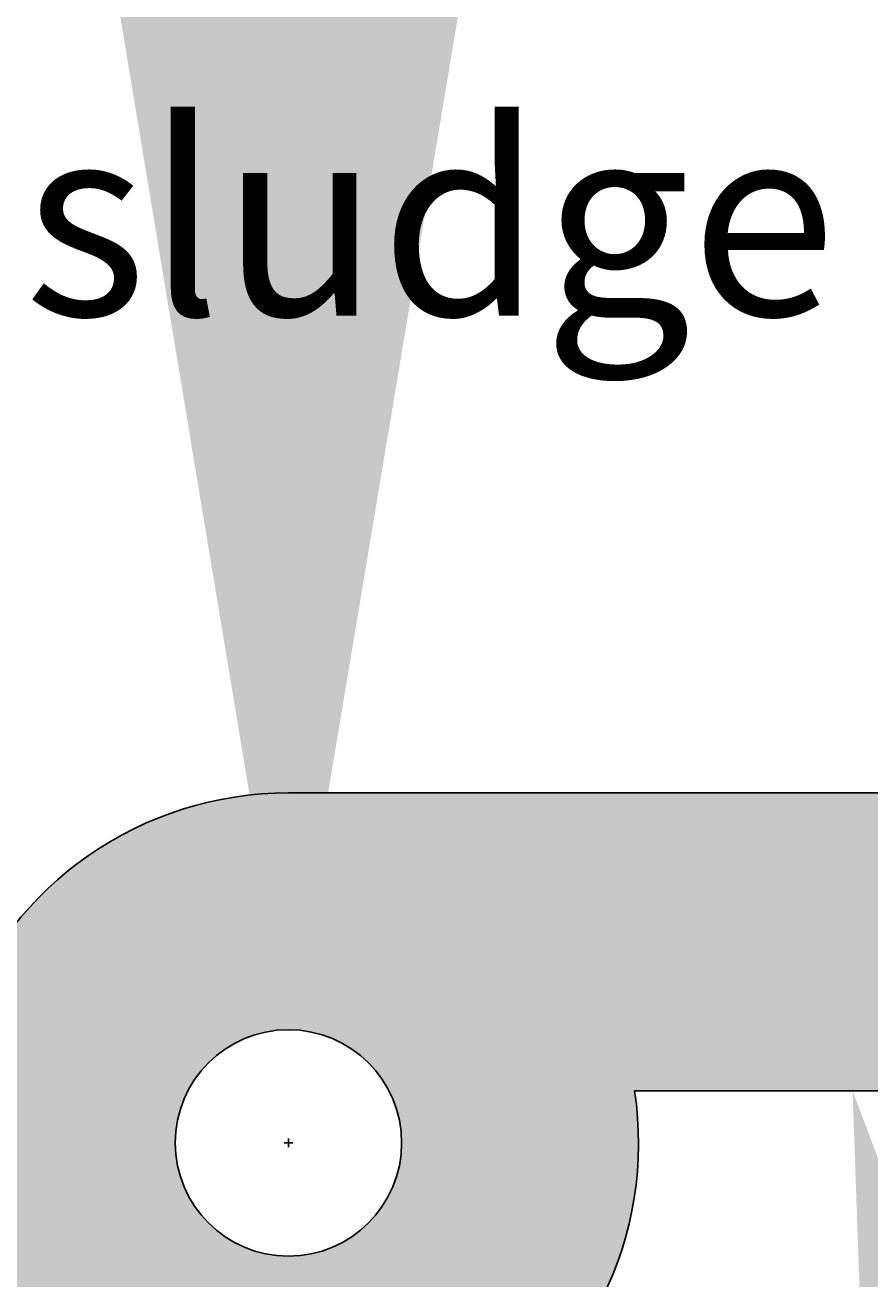
# Model space of a CAD drawing. Units: millimetres. Extents: x -22994 to 29398, y -19990 to 20176.
# Tile 12 of 135: x 41 to 58, y 26 to 52. Entities that reach past the tile are written whole.
import ezdxf
from ezdxf import colors
from ezdxf.entities.mleader import LeaderData, LeaderLine
from ezdxf.math import Vec2, Vec3

# ---------------------------------------------------------------- set-up
doc = ezdxf.new("R2010")
doc.units = ezdxf.units.MM
doc.header["$MEASUREMENT"] = 0
for name, color, linetype, lineweight in [('M-ANNO-TEXT', 7, 'Continuous', 25), ('M-DIMS', 2, 'Continuous', 18), ('M-EQPM', 7, 'Continuous', 25), ('M-EQPM-PATT', 7, 'Continuous', 18)]:
    doc.layers.add(name, color=color, linetype=linetype, lineweight=lineweight)
doc.styles.get("Standard").update_dxf_attribs({"font": 'arial.ttf'})
doc.dimstyles.get("Standard").update_dxf_attribs({"dimtxt": 0.18, "dimasz": 10000, "dimexe": 0.18, "dimexo": 0.0625, "dimgap": 0.09, "dimtad": 0, "dimtih": 1, "dimtoh": 1, "dimdec": 0, "dimzin": 0, "dimdsep": 46, "dimtxsty": 'Standard', "dimcen": 0.09, "dimadec": 0, "dimazin": 0, "dimtfac": 1, "dimtdec": 0, "dimtofl": 0, "dimtmove": 0, "dimatfit": 3, "dimfxl": 1, "dimtolj": 1, "dimtzin": 0, "dimlwd": 30, "dimarcsym": 0})

# ---------------------------------------------------------------- blocks, each defined once
blk = doc.blocks.new('*D2')
at = {"layer": 'Defpoints', "color": 0, "transparency": 16777216}
for p in [(6.677, 10.271), (290.852, 10.271), (290.852, -5.079)]:
    blk.add_point(p, dxfattribs=at)
at = {"layer": 'M-DIMS', "color": 0, "lineweight": -2, "transparency": 16777216}
for p, q in [((6.677, 10.209), (6.677, -5.259)), ((290.852, 10.209), (290.852, -5.259))]:
    blk.add_line(p, q, dxfattribs=at)
at = {"layer": 'M-DIMS', "color": 0, "lineweight": 30, "transparency": 16777216}
for p, q in [((-9993.323, -5.079), (-19993.323, -5.079)), ((10290.852, -5.079), (20290.852, -5.079))]:
    blk.add_line(p, q, dxfattribs=at)
at = {"layer": 'M-DIMS', "color": 0, "transparency": 16777216}
for points in [[(-9993.323, 1661.588), (-9993.323, -1671.745), (6.677, -5.079)], [(10290.852, 1661.588), (10290.852, -1671.745), (290.852, -5.079)]]:
    blk.add_solid(points, dxfattribs=at)
at = {"layer": 'M-DIMS', "color": 0, "transparency": 16777216, "insert": (148.765, -5.079), "char_height": 0.18, "attachment_point": 5}
blk.add_mtext('\\A1;284.2', dxfattribs=at)
blk = doc.blocks.new('*D3')
at = {"layer": 'Defpoints', "color": 0, "transparency": 16777216}
for p in [(110.265, 204.165), (110.265, 176.366), (95.833, 127.967)]:
    blk.add_point(p, dxfattribs=at)
at = {"layer": 'M-DIMS', "color": 0, "lineweight": -2, "transparency": 16777216}
for p, q in [((95.833, 128.03), (95.833, 204.345)), ((110.265, 176.429), (110.265, 204.345))]:
    blk.add_line(p, q, dxfattribs=at)
at = {"layer": 'M-DIMS', "color": 0, "lineweight": 30, "transparency": 16777216}
for p, q in [((-9904.167, 204.165), (-19904.167, 204.165)), ((10110.265, 204.165), (20110.265, 204.165))]:
    blk.add_line(p, q, dxfattribs=at)
at = {"layer": 'M-DIMS', "color": 0, "transparency": 16777216}
for points in [[(-9904.167, 1870.832), (-9904.167, -1462.501), (95.833, 204.165)], [(10110.265, 1870.832), (10110.265, -1462.501), (110.265, 204.165)]]:
    blk.add_solid(points, dxfattribs=at)
at = {"layer": 'M-DIMS', "color": 0, "transparency": 16777216, "insert": (103.049, 204.165), "char_height": 0.18, "attachment_point": 5}
blk.add_mtext('\\A1;14.432', dxfattribs=at)
blk = doc.blocks.new('*D4')
at = {"layer": 'Defpoints', "color": 0, "transparency": 16777216}
for p in [(116.265, 204.165), (110.265, 176.366), (116.265, 176.366)]:
    blk.add_point(p, dxfattribs=at)
at = {"layer": 'M-DIMS', "color": 0, "lineweight": -2, "transparency": 16777216}
for p, q in [((110.265, 176.429), (110.265, 204.345)), ((116.265, 176.429), (116.265, 204.345))]:
    blk.add_line(p, q, dxfattribs=at)
at = {"layer": 'M-DIMS', "color": 0, "lineweight": 30, "transparency": 16777216}
for p, q in [((-9889.735, 204.165), (-19889.735, 204.165)), ((10116.265, 204.165), (20116.265, 204.165))]:
    blk.add_line(p, q, dxfattribs=at)
at = {"layer": 'M-DIMS', "color": 0, "transparency": 16777216}
for points in [[(-9889.735, 1870.832), (-9889.735, -1462.501), (110.265, 204.165)], [(10116.265, 1870.832), (10116.265, -1462.501), (116.265, 204.165)]]:
    blk.add_solid(points, dxfattribs=at)
at = {"layer": 'M-DIMS', "color": 0, "transparency": 16777216, "insert": (113.265, 204.165), "char_height": 0.18, "attachment_point": 5}
blk.add_mtext('\\A1;6', dxfattribs=at)
blk = doc.blocks.new('*D5')
at = {"layer": 'Defpoints', "color": 0, "transparency": 16777216}
for p in [(181.265, 204.165), (116.265, 176.366), (181.265, 176.366)]:
    blk.add_point(p, dxfattribs=at)
at = {"layer": 'M-DIMS', "color": 0, "lineweight": -2, "transparency": 16777216}
for p, q in [((116.265, 176.429), (116.265, 204.345)), ((181.265, 176.429), (181.265, 204.345))]:
    blk.add_line(p, q, dxfattribs=at)
at = {"layer": 'M-DIMS', "color": 0, "lineweight": 30, "transparency": 16777216}
for p, q in [((-9883.735, 204.165), (-19883.735, 204.165)), ((10181.265, 204.165), (20181.265, 204.165))]:
    blk.add_line(p, q, dxfattribs=at)
at = {"layer": 'M-DIMS', "color": 0, "transparency": 16777216}
for points in [[(-9883.735, 1870.832), (-9883.735, -1462.501), (116.265, 204.165)], [(10181.265, 1870.832), (10181.265, -1462.501), (181.265, 204.165)]]:
    blk.add_solid(points, dxfattribs=at)
at = {"layer": 'M-DIMS', "color": 0, "transparency": 16777216, "insert": (148.765, 204.165), "char_height": 0.18, "attachment_point": 5}
blk.add_mtext('\\A1;65', dxfattribs=at)
blk = doc.blocks.new('*D6')
at = {"layer": 'Defpoints', "color": 0, "transparency": 16777216}
for p in [(187.265, 204.165), (181.265, 176.366), (187.265, 176.366)]:
    blk.add_point(p, dxfattribs=at)
at = {"layer": 'M-DIMS', "color": 0, "lineweight": -2, "transparency": 16777216}
for p, q in [((181.265, 176.429), (181.265, 204.345)), ((187.265, 176.429), (187.265, 204.345))]:
    blk.add_line(p, q, dxfattribs=at)
at = {"layer": 'M-DIMS', "color": 0, "lineweight": 30, "transparency": 16777216}
for p, q in [((-9818.735, 204.165), (-19818.735, 204.165)), ((10187.265, 204.165), (20187.265, 204.165))]:
    blk.add_line(p, q, dxfattribs=at)
at = {"layer": 'M-DIMS', "color": 0, "transparency": 16777216}
for points in [[(-9818.735, 1870.832), (-9818.735, -1462.501), (181.265, 204.165)], [(10187.265, 1870.832), (10187.265, -1462.501), (187.265, 204.165)]]:
    blk.add_solid(points, dxfattribs=at)
at = {"layer": 'M-DIMS', "color": 0, "transparency": 16777216, "insert": (184.265, 204.165), "char_height": 0.18, "attachment_point": 5}
blk.add_mtext('\\A1;6', dxfattribs=at)
blk = doc.blocks.new('*D7')
at = {"layer": 'Defpoints', "color": 0, "transparency": 16777216}
for p in [(201.697, 204.165), (187.265, 176.366), (201.697, 127.967)]:
    blk.add_point(p, dxfattribs=at)
at = {"layer": 'M-DIMS', "color": 0, "lineweight": -2, "transparency": 16777216}
for p, q in [((187.265, 176.429), (187.265, 204.345)), ((201.697, 128.03), (201.697, 204.345))]:
    blk.add_line(p, q, dxfattribs=at)
at = {"layer": 'M-DIMS', "color": 0, "lineweight": 30, "transparency": 16777216}
for p, q in [((-9812.735, 204.165), (-19812.735, 204.165)), ((10201.697, 204.165), (20201.697, 204.165))]:
    blk.add_line(p, q, dxfattribs=at)
at = {"layer": 'M-DIMS', "color": 0, "transparency": 16777216}
for points in [[(-9812.735, 1870.832), (-9812.735, -1462.501), (187.265, 204.165)], [(10201.697, 1870.832), (10201.697, -1462.501), (201.697, 204.165)]]:
    blk.add_solid(points, dxfattribs=at)
at = {"layer": 'M-DIMS', "color": 0, "transparency": 16777216, "insert": (194.481, 204.165), "char_height": 0.18, "attachment_point": 5}
blk.add_mtext('\\A1;14.432', dxfattribs=at)
blk = doc.blocks.new('*D8')
at = {"layer": 'Defpoints', "color": 0, "transparency": 16777216}
for p in [(227.648, 204.165), (227.648, 146.73), (201.697, 127.967)]:
    blk.add_point(p, dxfattribs=at)
at = {"layer": 'M-DIMS', "color": 0, "lineweight": -2, "transparency": 16777216}
for p, q in [((201.697, 128.03), (201.697, 204.345)), ((227.648, 146.792), (227.648, 204.345))]:
    blk.add_line(p, q, dxfattribs=at)
at = {"layer": 'M-DIMS', "color": 0, "lineweight": 30, "transparency": 16777216}
for p, q in [((-9798.303, 204.165), (-19798.303, 204.165)), ((10227.648, 204.165), (20227.648, 204.165))]:
    blk.add_line(p, q, dxfattribs=at)
at = {"layer": 'M-DIMS', "color": 0, "transparency": 16777216}
for points in [[(-9798.303, 1870.832), (-9798.303, -1462.501), (201.697, 204.165)], [(10227.648, 1870.832), (10227.648, -1462.501), (227.648, 204.165)]]:
    blk.add_solid(points, dxfattribs=at)
at = {"layer": 'M-DIMS', "color": 0, "transparency": 16777216, "insert": (214.673, 204.165), "char_height": 0.18, "attachment_point": 5}
blk.add_mtext('\\A1;25.95', dxfattribs=at)
blk = doc.blocks.new('*D9')
at = {"layer": 'Defpoints', "color": 0, "transparency": 16777216}
for p in [(187.265, 176.366), (306.202, 176.366), (290.852, 10.271)]:
    blk.add_point(p, dxfattribs=at)
at = {"layer": 'M-DIMS', "color": 0, "lineweight": 30, "transparency": 16777216}
for p, q in [((306.202, 10176.366), (306.202, 20176.366)), ((306.202, -9989.729), (306.202, -19989.729))]:
    blk.add_line(p, q, dxfattribs=at)
at = {"layer": 'M-DIMS', "color": 0, "lineweight": -2, "transparency": 16777216}
for p, q in [((187.327, 176.366), (306.382, 176.366)), ((290.915, 10.271), (306.382, 10.271))]:
    blk.add_line(p, q, dxfattribs=at)
at = {"layer": 'M-DIMS', "color": 0, "transparency": 16777216}
for points in [[(-1360.465, 10176.366), (1972.869, 10176.366), (306.202, 176.366)], [(-1360.465, -9989.729), (1972.869, -9989.729), (306.202, 10.271)]]:
    blk.add_solid(points, dxfattribs=at)
at = {"layer": 'M-DIMS', "color": 0, "transparency": 16777216, "insert": (306.202, 93.319), "char_height": 0.18, "attachment_point": 5}
blk.add_mtext('\\A1;166.1', dxfattribs=at)
blk = doc.blocks.new('*D10')
at = {"layer": 'Defpoints', "color": 0, "transparency": 16777216}
for p in [(125.65, 136.071), (133.346, 136.071), (133.346, -5.079)]:
    blk.add_point(p, dxfattribs=at)
at = {"layer": 'M-DIMS', "color": 0, "lineweight": -2, "transparency": 16777216}
for p, q in [((125.65, 136.009), (125.65, -5.259)), ((133.346, 136.009), (133.346, -5.259))]:
    blk.add_line(p, q, dxfattribs=at)
at = {"layer": 'M-DIMS', "color": 0, "lineweight": 30, "transparency": 16777216}
for p, q in [((-9874.35, -5.079), (-19874.35, -5.079)), ((10133.346, -5.079), (20133.346, -5.079))]:
    blk.add_line(p, q, dxfattribs=at)
at = {"layer": 'M-DIMS', "color": 0, "transparency": 16777216}
for points in [[(-9874.35, 1661.588), (-9874.35, -1671.745), (125.65, -5.079)], [(10133.346, 1661.588), (10133.346, -1671.745), (133.346, -5.079)]]:
    blk.add_solid(points, dxfattribs=at)
at = {"layer": 'M-DIMS', "color": 0, "transparency": 16777216, "insert": (129.498, -5.079), "char_height": 0.18, "attachment_point": 5}
blk.add_mtext('\\A1;7.696', dxfattribs=at)
blk = doc.blocks.new('*D11')
at = {"layer": 'Defpoints', "color": 0, "transparency": 16777216}
for p in [(133.346, 136.071), (135.65, 136.071), (135.65, -5.079)]:
    blk.add_point(p, dxfattribs=at)
at = {"layer": 'M-DIMS', "color": 0, "lineweight": -2, "transparency": 16777216}
for p, q in [((133.346, 136.009), (133.346, -5.259)), ((135.65, 136.009), (135.65, -5.259))]:
    blk.add_line(p, q, dxfattribs=at)
at = {"layer": 'M-DIMS', "color": 0, "lineweight": 30, "transparency": 16777216}
for p, q in [((-9866.654, -5.079), (-19866.654, -5.079)), ((10135.65, -5.079), (20135.65, -5.079))]:
    blk.add_line(p, q, dxfattribs=at)
at = {"layer": 'M-DIMS', "color": 0, "transparency": 16777216}
for points in [[(-9866.654, 1661.588), (-9866.654, -1671.745), (133.346, -5.079)], [(10135.65, 1661.588), (10135.65, -1671.745), (135.65, -5.079)]]:
    blk.add_solid(points, dxfattribs=at)
at = {"layer": 'M-DIMS', "color": 0, "transparency": 16777216, "insert": (134.498, -5.079), "char_height": 0.18, "attachment_point": 5}
blk.add_mtext('\\A1;2.304', dxfattribs=at)
blk = doc.blocks.new('*D12')
at = {"layer": 'Defpoints', "color": 0, "transparency": 16777216}
for p in [(135.65, 136.071), (145.65, 136.071), (145.65, -5.079)]:
    blk.add_point(p, dxfattribs=at)
at = {"layer": 'M-DIMS', "color": 0, "lineweight": -2, "transparency": 16777216}
for p, q in [((135.65, 136.009), (135.65, -5.259)), ((145.65, 136.009), (145.65, -5.259))]:
    blk.add_line(p, q, dxfattribs=at)
at = {"layer": 'M-DIMS', "color": 0, "lineweight": 30, "transparency": 16777216}
for p, q in [((-9864.35, -5.079), (-19864.35, -5.079)), ((10145.65, -5.079), (20145.65, -5.079))]:
    blk.add_line(p, q, dxfattribs=at)
at = {"layer": 'M-DIMS', "color": 0, "transparency": 16777216}
for points in [[(-9864.35, 1661.588), (-9864.35, -1671.745), (135.65, -5.079)], [(10145.65, 1661.588), (10145.65, -1671.745), (145.65, -5.079)]]:
    blk.add_solid(points, dxfattribs=at)
at = {"layer": 'M-DIMS', "color": 0, "transparency": 16777216, "insert": (140.65, -5.079), "char_height": 0.18, "attachment_point": 5}
blk.add_mtext('\\A1;10', dxfattribs=at)
blk = doc.blocks.new('*D13')
at = {"layer": 'Defpoints', "color": 0, "transparency": 16777216}
for p in [(145.65, 136.071), (155.65, 136.071), (155.65, -5.079)]:
    blk.add_point(p, dxfattribs=at)
at = {"layer": 'M-DIMS', "color": 0, "lineweight": -2, "transparency": 16777216}
for p, q in [((145.65, 136.009), (145.65, -5.259)), ((155.65, 136.009), (155.65, -5.259))]:
    blk.add_line(p, q, dxfattribs=at)
at = {"layer": 'M-DIMS', "color": 0, "lineweight": 30, "transparency": 16777216}
for p, q in [((-9854.35, -5.079), (-19854.35, -5.079)), ((10155.65, -5.079), (20155.65, -5.079))]:
    blk.add_line(p, q, dxfattribs=at)
at = {"layer": 'M-DIMS', "color": 0, "transparency": 16777216}
for points in [[(-9854.35, 1661.588), (-9854.35, -1671.745), (145.65, -5.079)], [(10155.65, 1661.588), (10155.65, -1671.745), (155.65, -5.079)]]:
    blk.add_solid(points, dxfattribs=at)
at = {"layer": 'M-DIMS', "color": 0, "transparency": 16777216, "insert": (150.65, -5.079), "char_height": 0.18, "attachment_point": 5}
blk.add_mtext('\\A1;10', dxfattribs=at)
blk = doc.blocks.new('*D14')
at = {"layer": 'Defpoints', "color": 0, "transparency": 16777216}
for p in [(155.65, 136.071), (165.65, 136.071), (165.65, -5.079)]:
    blk.add_point(p, dxfattribs=at)
at = {"layer": 'M-DIMS', "color": 0, "lineweight": -2, "transparency": 16777216}
for p, q in [((155.65, 136.009), (155.65, -5.259)), ((165.65, 136.009), (165.65, -5.259))]:
    blk.add_line(p, q, dxfattribs=at)
at = {"layer": 'M-DIMS', "color": 0, "lineweight": 30, "transparency": 16777216}
for p, q in [((-9844.35, -5.079), (-19844.35, -5.079)), ((10165.65, -5.079), (20165.65, -5.079))]:
    blk.add_line(p, q, dxfattribs=at)
at = {"layer": 'M-DIMS', "color": 0, "transparency": 16777216}
for points in [[(-9844.35, 1661.588), (-9844.35, -1671.745), (155.65, -5.079)], [(10165.65, 1661.588), (10165.65, -1671.745), (165.65, -5.079)]]:
    blk.add_solid(points, dxfattribs=at)
at = {"layer": 'M-DIMS', "color": 0, "transparency": 16777216, "insert": (160.65, -5.079), "char_height": 0.18, "attachment_point": 5}
blk.add_mtext('\\A1;10', dxfattribs=at)
blk = doc.blocks.new('*D15')
at = {"layer": 'Defpoints', "color": 0, "transparency": 16777216}
for p in [(173.346, 154.788), (173.346, 136.071), (306.202, 136.071)]:
    blk.add_point(p, dxfattribs=at)
at = {"layer": 'M-DIMS', "color": 0, "lineweight": 30, "transparency": 16777216}
for p, q in [((306.202, 10154.788), (306.202, 20154.788)), ((306.202, -9863.929), (306.202, -19863.929))]:
    blk.add_line(p, q, dxfattribs=at)
at = {"layer": 'M-DIMS', "color": 0, "lineweight": -2, "transparency": 16777216}
for p, q in [((173.408, 154.788), (306.382, 154.788)), ((173.408, 136.071), (306.382, 136.071))]:
    blk.add_line(p, q, dxfattribs=at)
at = {"layer": 'M-DIMS', "color": 0, "transparency": 16777216}
for points in [[(-1360.465, 10154.788), (1972.869, 10154.788), (306.202, 154.788)], [(-1360.465, -9863.929), (1972.869, -9863.929), (306.202, 136.071)]]:
    blk.add_solid(points, dxfattribs=at)
at = {"layer": 'M-DIMS', "color": 0, "transparency": 16777216, "insert": (306.202, 145.43), "char_height": 0.18, "attachment_point": 5}
blk.add_mtext('\\A1;18.717', dxfattribs=at)
blk = doc.blocks.new('*D16')
at = {"layer": 'Defpoints', "color": 0, "transparency": 16777216}
for p in [(120.17, 204.165), (110.466, 48.035), (120.17, 48.035)]:
    blk.add_point(p, dxfattribs=at)
at = {"layer": 'M-DIMS', "color": 0, "lineweight": -2, "transparency": 16777216}
for p, q in [((110.466, 48.097), (110.466, 204.345)), ((120.17, 48.097), (120.17, 204.345))]:
    blk.add_line(p, q, dxfattribs=at)
at = {"layer": 'M-DIMS', "color": 0, "lineweight": 30, "transparency": 16777216}
for p, q in [((-9889.534, 204.165), (-19889.534, 204.165)), ((10120.17, 204.165), (20120.17, 204.165))]:
    blk.add_line(p, q, dxfattribs=at)
at = {"layer": 'M-DIMS', "color": 0, "transparency": 16777216}
for points in [[(-9889.534, 1870.832), (-9889.534, -1462.501), (110.466, 204.165)], [(10120.17, 1870.832), (10120.17, -1462.501), (120.17, 204.165)]]:
    blk.add_solid(points, dxfattribs=at)
at = {"layer": 'M-DIMS', "color": 0, "transparency": 16777216, "insert": (115.318, 204.165), "char_height": 0.18, "attachment_point": 5}
blk.add_mtext('\\A1;9.704', dxfattribs=at)
blk = doc.blocks.new('*D17')
at = {"layer": 'Defpoints', "color": 0, "transparency": 16777216}
for p in [(126.17, 204.165), (120.17, 48.035), (126.17, 48.035)]:
    blk.add_point(p, dxfattribs=at)
at = {"layer": 'M-DIMS', "color": 0, "lineweight": -2, "transparency": 16777216}
for p, q in [((120.17, 48.097), (120.17, 204.345)), ((126.17, 48.097), (126.17, 204.345))]:
    blk.add_line(p, q, dxfattribs=at)
at = {"layer": 'M-DIMS', "color": 0, "lineweight": 30, "transparency": 16777216}
for p, q in [((-9879.83, 204.165), (-19879.83, 204.165)), ((10126.17, 204.165), (20126.17, 204.165))]:
    blk.add_line(p, q, dxfattribs=at)
at = {"layer": 'M-DIMS', "color": 0, "transparency": 16777216}
for points in [[(-9879.83, 1870.832), (-9879.83, -1462.501), (120.17, 204.165)], [(10126.17, 1870.832), (10126.17, -1462.501), (126.17, 204.165)]]:
    blk.add_solid(points, dxfattribs=at)
at = {"layer": 'M-DIMS', "color": 0, "transparency": 16777216, "insert": (123.17, 204.165), "char_height": 0.18, "attachment_point": 5}
blk.add_mtext('\\A1;6', dxfattribs=at)
blk = doc.blocks.new('*D18')
at = {"layer": 'Defpoints', "color": 0, "transparency": 16777216}
for p in [(132.17, 204.165), (126.17, 48.035), (132.17, 48.035)]:
    blk.add_point(p, dxfattribs=at)
at = {"layer": 'M-DIMS', "color": 0, "lineweight": -2, "transparency": 16777216}
for p, q in [((126.17, 48.097), (126.17, 204.345)), ((132.17, 48.097), (132.17, 204.345))]:
    blk.add_line(p, q, dxfattribs=at)
at = {"layer": 'M-DIMS', "color": 0, "lineweight": 30, "transparency": 16777216}
for p, q in [((-9873.83, 204.165), (-19873.83, 204.165)), ((10132.17, 204.165), (20132.17, 204.165))]:
    blk.add_line(p, q, dxfattribs=at)
at = {"layer": 'M-DIMS', "color": 0, "transparency": 16777216}
for points in [[(-9873.83, 1870.832), (-9873.83, -1462.501), (126.17, 204.165)], [(10132.17, 1870.832), (10132.17, -1462.501), (132.17, 204.165)]]:
    blk.add_solid(points, dxfattribs=at)
at = {"layer": 'M-DIMS', "color": 0, "transparency": 16777216, "insert": (129.17, 204.165), "char_height": 0.18, "attachment_point": 5}
blk.add_mtext('\\A1;6', dxfattribs=at)
blk = doc.blocks.new('*D19')
at = {"layer": 'Defpoints', "color": 0, "transparency": 16777216}
for p in [(138.17, 204.165), (132.17, 48.035), (138.17, 48.035)]:
    blk.add_point(p, dxfattribs=at)
at = {"layer": 'M-DIMS', "color": 0, "lineweight": -2, "transparency": 16777216}
for p, q in [((132.17, 48.097), (132.17, 204.345)), ((138.17, 48.097), (138.17, 204.345))]:
    blk.add_line(p, q, dxfattribs=at)
at = {"layer": 'M-DIMS', "color": 0, "lineweight": 30, "transparency": 16777216}
for p, q in [((-9867.83, 204.165), (-19867.83, 204.165)), ((10138.17, 204.165), (20138.17, 204.165))]:
    blk.add_line(p, q, dxfattribs=at)
at = {"layer": 'M-DIMS', "color": 0, "transparency": 16777216}
for points in [[(-9867.83, 1870.832), (-9867.83, -1462.501), (132.17, 204.165)], [(10138.17, 1870.832), (10138.17, -1462.501), (138.17, 204.165)]]:
    blk.add_solid(points, dxfattribs=at)
at = {"layer": 'M-DIMS', "color": 0, "transparency": 16777216, "insert": (135.17, 204.165), "char_height": 0.18, "attachment_point": 5}
blk.add_mtext('\\A1;6', dxfattribs=at)
blk = doc.blocks.new('*D20')
at = {"layer": 'Defpoints', "color": 0, "transparency": 16777216}
for p in [(144.17, 204.165), (138.17, 48.035), (144.17, 48.035)]:
    blk.add_point(p, dxfattribs=at)
at = {"layer": 'M-DIMS', "color": 0, "lineweight": -2, "transparency": 16777216}
for p, q in [((138.17, 48.097), (138.17, 204.345)), ((144.17, 48.097), (144.17, 204.345))]:
    blk.add_line(p, q, dxfattribs=at)
at = {"layer": 'M-DIMS', "color": 0, "lineweight": 30, "transparency": 16777216}
for p, q in [((-9861.83, 204.165), (-19861.83, 204.165)), ((10144.17, 204.165), (20144.17, 204.165))]:
    blk.add_line(p, q, dxfattribs=at)
at = {"layer": 'M-DIMS', "color": 0, "transparency": 16777216}
for points in [[(-9861.83, 1870.832), (-9861.83, -1462.501), (138.17, 204.165)], [(10144.17, 1870.832), (10144.17, -1462.501), (144.17, 204.165)]]:
    blk.add_solid(points, dxfattribs=at)
at = {"layer": 'M-DIMS', "color": 0, "transparency": 16777216, "insert": (141.17, 204.165), "char_height": 0.18, "attachment_point": 5}
blk.add_mtext('\\A1;6', dxfattribs=at)
blk = doc.blocks.new('*D21')
at = {"layer": 'Defpoints', "color": 0, "transparency": 16777216}
for p in [(149.116, 204.165), (144.17, 48.035), (149.116, 48.035)]:
    blk.add_point(p, dxfattribs=at)
at = {"layer": 'M-DIMS', "color": 0, "lineweight": -2, "transparency": 16777216}
for p, q in [((144.17, 48.097), (144.17, 204.345)), ((149.116, 48.097), (149.116, 204.345))]:
    blk.add_line(p, q, dxfattribs=at)
at = {"layer": 'M-DIMS', "color": 0, "lineweight": 30, "transparency": 16777216}
for p, q in [((-9855.83, 204.165), (-19855.83, 204.165)), ((10149.116, 204.165), (20149.116, 204.165))]:
    blk.add_line(p, q, dxfattribs=at)
at = {"layer": 'M-DIMS', "color": 0, "transparency": 16777216}
for points in [[(-9855.83, 1870.832), (-9855.83, -1462.501), (144.17, 204.165)], [(10149.116, 1870.832), (10149.116, -1462.501), (149.116, 204.165)]]:
    blk.add_solid(points, dxfattribs=at)
at = {"layer": 'M-DIMS', "color": 0, "transparency": 16777216, "insert": (146.643, 204.165), "char_height": 0.18, "attachment_point": 5}
blk.add_mtext('\\A1;4.945', dxfattribs=at)
blk = doc.blocks.new('*D22')
at = {"layer": 'Defpoints', "color": 0, "transparency": 16777216}
for p in [(149.116, 30.99), (155.116, 30.99), (155.116, -5.079)]:
    blk.add_point(p, dxfattribs=at)
at = {"layer": 'M-DIMS', "color": 0, "lineweight": -2, "transparency": 16777216}
for p, q in [((149.116, 30.927), (149.116, -5.259)), ((155.116, 30.927), (155.116, -5.259))]:
    blk.add_line(p, q, dxfattribs=at)
at = {"layer": 'M-DIMS', "color": 0, "lineweight": 30, "transparency": 16777216}
for p, q in [((-9850.884, -5.079), (-19850.884, -5.079)), ((10155.116, -5.079), (20155.116, -5.079))]:
    blk.add_line(p, q, dxfattribs=at)
at = {"layer": 'M-DIMS', "color": 0, "transparency": 16777216}
for points in [[(-9850.884, 1661.588), (-9850.884, -1671.745), (149.116, -5.079)], [(10155.116, 1661.588), (10155.116, -1671.745), (155.116, -5.079)]]:
    blk.add_solid(points, dxfattribs=at)
at = {"layer": 'M-DIMS', "color": 0, "transparency": 16777216, "insert": (152.116, -5.079), "char_height": 0.18, "attachment_point": 5}
blk.add_mtext('\\A1;6', dxfattribs=at)
blk = doc.blocks.new('*D23')
at = {"layer": 'Defpoints', "color": 0, "transparency": 16777216}
for p in [(155.116, 30.99), (161.116, 30.99), (161.116, -5.079)]:
    blk.add_point(p, dxfattribs=at)
at = {"layer": 'M-DIMS', "color": 0, "lineweight": -2, "transparency": 16777216}
for p, q in [((155.116, 30.927), (155.116, -5.259)), ((161.116, 30.927), (161.116, -5.259))]:
    blk.add_line(p, q, dxfattribs=at)
at = {"layer": 'M-DIMS', "color": 0, "lineweight": 30, "transparency": 16777216}
for p, q in [((-9844.884, -5.079), (-19844.884, -5.079)), ((10161.116, -5.079), (20161.116, -5.079))]:
    blk.add_line(p, q, dxfattribs=at)
at = {"layer": 'M-DIMS', "color": 0, "transparency": 16777216}
for points in [[(-9844.884, 1661.588), (-9844.884, -1671.745), (155.116, -5.079)], [(10161.116, 1661.588), (10161.116, -1671.745), (161.116, -5.079)]]:
    blk.add_solid(points, dxfattribs=at)
at = {"layer": 'M-DIMS', "color": 0, "transparency": 16777216, "insert": (158.116, -5.079), "char_height": 0.18, "attachment_point": 5}
blk.add_mtext('\\A1;6', dxfattribs=at)
blk = doc.blocks.new('*D24')
at = {"layer": 'Defpoints', "color": 0, "transparency": 16777216}
for p in [(161.116, 30.99), (166.439, 30.99), (166.439, -5.079)]:
    blk.add_point(p, dxfattribs=at)
at = {"layer": 'M-DIMS', "color": 0, "lineweight": -2, "transparency": 16777216}
for p, q in [((161.116, 30.927), (161.116, -5.259)), ((166.439, 30.927), (166.439, -5.259))]:
    blk.add_line(p, q, dxfattribs=at)
at = {"layer": 'M-DIMS', "color": 0, "lineweight": 30, "transparency": 16777216}
for p, q in [((-9838.884, -5.079), (-19838.884, -5.079)), ((10166.439, -5.079), (20166.439, -5.079))]:
    blk.add_line(p, q, dxfattribs=at)
at = {"layer": 'M-DIMS', "color": 0, "transparency": 16777216}
for points in [[(-9838.884, 1661.588), (-9838.884, -1671.745), (161.116, -5.079)], [(10166.439, 1661.588), (10166.439, -1671.745), (166.439, -5.079)]]:
    blk.add_solid(points, dxfattribs=at)
at = {"layer": 'M-DIMS', "color": 0, "transparency": 16777216, "insert": (163.777, -5.079), "char_height": 0.18, "attachment_point": 5}
blk.add_mtext('\\A1;5.323', dxfattribs=at)
blk = doc.blocks.new('*D25')
at = {"layer": 'Defpoints', "color": 0, "transparency": 16777216}
for p in [(166.439, 30.99), (172.439, 30.99), (172.439, -5.079)]:
    blk.add_point(p, dxfattribs=at)
at = {"layer": 'M-DIMS', "color": 0, "lineweight": -2, "transparency": 16777216}
for p, q in [((166.439, 30.927), (166.439, -5.259)), ((172.439, 30.927), (172.439, -5.259))]:
    blk.add_line(p, q, dxfattribs=at)
at = {"layer": 'M-DIMS', "color": 0, "lineweight": 30, "transparency": 16777216}
for p, q in [((-9833.561, -5.079), (-19833.561, -5.079)), ((10172.439, -5.079), (20172.439, -5.079))]:
    blk.add_line(p, q, dxfattribs=at)
at = {"layer": 'M-DIMS', "color": 0, "transparency": 16777216}
for points in [[(-9833.561, 1661.588), (-9833.561, -1671.745), (166.439, -5.079)], [(10172.439, 1661.588), (10172.439, -1671.745), (172.439, -5.079)]]:
    blk.add_solid(points, dxfattribs=at)
at = {"layer": 'M-DIMS', "color": 0, "transparency": 16777216, "insert": (169.439, -5.079), "char_height": 0.18, "attachment_point": 5}
blk.add_mtext('\\A1;6', dxfattribs=at)
blk = doc.blocks.new('*D26')
at = {"layer": 'Defpoints', "color": 0, "transparency": 16777216}
for p in [(172.439, 30.99), (178.439, 30.99), (178.439, -5.079)]:
    blk.add_point(p, dxfattribs=at)
at = {"layer": 'M-DIMS', "color": 0, "lineweight": -2, "transparency": 16777216}
for p, q in [((172.439, 30.927), (172.439, -5.259)), ((178.439, 30.927), (178.439, -5.259))]:
    blk.add_line(p, q, dxfattribs=at)
at = {"layer": 'M-DIMS', "color": 0, "lineweight": 30, "transparency": 16777216}
for p, q in [((-9827.561, -5.079), (-19827.561, -5.079)), ((10178.439, -5.079), (20178.439, -5.079))]:
    blk.add_line(p, q, dxfattribs=at)
at = {"layer": 'M-DIMS', "color": 0, "transparency": 16777216}
for points in [[(-9827.561, 1661.588), (-9827.561, -1671.745), (172.439, -5.079)], [(10178.439, 1661.588), (10178.439, -1671.745), (178.439, -5.079)]]:
    blk.add_solid(points, dxfattribs=at)
at = {"layer": 'M-DIMS', "color": 0, "transparency": 16777216, "insert": (175.439, -5.079), "char_height": 0.18, "attachment_point": 5}
blk.add_mtext('\\A1;6', dxfattribs=at)
blk = doc.blocks.new('*D27')
at = {"layer": 'Defpoints', "color": 0, "transparency": 16777216}
for p in [(178.439, 30.99), (188.117, 30.99), (188.117, -5.079)]:
    blk.add_point(p, dxfattribs=at)
at = {"layer": 'M-DIMS', "color": 0, "lineweight": -2, "transparency": 16777216}
for p, q in [((178.439, 30.927), (178.439, -5.259)), ((188.117, 30.927), (188.117, -5.259))]:
    blk.add_line(p, q, dxfattribs=at)
at = {"layer": 'M-DIMS', "color": 0, "lineweight": 30, "transparency": 16777216}
for p, q in [((-9821.561, -5.079), (-19821.561, -5.079)), ((10188.117, -5.079), (20188.117, -5.079))]:
    blk.add_line(p, q, dxfattribs=at)
at = {"layer": 'M-DIMS', "color": 0, "transparency": 16777216}
for points in [[(-9821.561, 1661.588), (-9821.561, -1671.745), (178.439, -5.079)], [(10188.117, 1661.588), (10188.117, -1671.745), (188.117, -5.079)]]:
    blk.add_solid(points, dxfattribs=at)
at = {"layer": 'M-DIMS', "color": 0, "transparency": 16777216, "insert": (183.278, -5.079), "char_height": 0.18, "attachment_point": 5}
blk.add_mtext('\\A1;9.679', dxfattribs=at)
blk = doc.blocks.new('*D28')
at = {"layer": 'Defpoints', "color": 0, "transparency": 16777216}
for p in [(188.117, 48.035), (306.202, 48.035), (188.117, 30.99)]:
    blk.add_point(p, dxfattribs=at)
at = {"layer": 'M-DIMS', "color": 0, "lineweight": 30, "transparency": 16777216}
for p, q in [((306.202, 10048.035), (306.202, 20048.035)), ((306.202, -9969.01), (306.202, -19969.01))]:
    blk.add_line(p, q, dxfattribs=at)
at = {"layer": 'M-DIMS', "color": 0, "lineweight": -2, "transparency": 16777216}
for p, q in [((188.18, 48.035), (306.382, 48.035)), ((188.18, 30.99), (306.382, 30.99))]:
    blk.add_line(p, q, dxfattribs=at)
at = {"layer": 'M-DIMS', "color": 0, "transparency": 16777216}
for points in [[(-1360.465, 10048.035), (1972.869, 10048.035), (306.202, 48.035)], [(-1360.465, -9969.01), (1972.869, -9969.01), (306.202, 30.99)]]:
    blk.add_solid(points, dxfattribs=at)
at = {"layer": 'M-DIMS', "color": 0, "transparency": 16777216, "insert": (306.202, 39.512), "char_height": 0.18, "attachment_point": 5}
blk.add_mtext('\\A1;17.045', dxfattribs=at)
blk = doc.blocks.new('*D29')
at = {"layer": 'Defpoints', "color": 0, "transparency": 16777216}
for p in [(36.801, 80.045), (64.03, 80.045)]:
    blk.add_point(p, dxfattribs=at)
at = {"layer": 'M-DIMS', "color": 0, "lineweight": -2, "transparency": 16777216}
for p, q in [((50.415, 79.955), (50.415, 80.135)), ((50.325, 80.045), (50.505, 80.045))]:
    blk.add_line(p, q, dxfattribs=at)
at = {"layer": 'M-DIMS', "color": 0, "lineweight": 30, "transparency": 16777216}
blk.add_line((20064.03, 80.03), (10064.03, 80.038), dxfattribs=at)
at = {"layer": 'M-DIMS', "color": 0, "transparency": 16777216}
blk.add_solid([(10064.031, 1746.704), (10064.028, -1586.629), (64.03, 80.045)], dxfattribs=at)
at = {"layer": 'M-DIMS', "color": 0, "transparency": 16777216, "insert": (20064.521, 80.03), "char_height": 0.18, "attachment_point": 5}
blk.add_mtext('\\A1;∅27.23', dxfattribs=at)
blk = doc.blocks.new('*D32')
at = {"layer": 'Defpoints', "color": 0, "transparency": 16777216}
for p in [(57.164, 118.614), (52.413, 113.093)]:
    blk.add_point(p, dxfattribs=at)
at = {"layer": 'M-DIMS', "color": 0, "lineweight": -2, "transparency": 16777216}
for p, q in [((57.074, 118.614), (57.254, 118.614)), ((57.164, 118.524), (57.164, 118.704))]:
    blk.add_line(p, q, dxfattribs=at)
at = {"layer": 'M-DIMS', "color": 0, "lineweight": 30, "transparency": 16777216}
for p, q in [((-12992.534, -15047.031), (-6470.06, -7466.969)), ((-22992.534, -15047.031), (-12992.534, -15047.031))]:
    blk.add_line(p, q, dxfattribs=at)
at = {"layer": 'M-DIMS', "color": 0, "transparency": 16777216}
blk.add_solid([(-7733.404, -6379.89), (-5206.717, -8554.048), (52.413, 113.093)], dxfattribs=at)
at = {"layer": 'M-DIMS', "color": 0, "transparency": 16777216, "insert": (-22993.208, -15047.031), "char_height": 0.18, "attachment_point": 5}
blk.add_mtext('\\A1;2X R7.284', dxfattribs=at)
blk = doc.blocks.new('*D36')
at = {"layer": 'Defpoints', "color": 0, "transparency": 16777216}
for p in [(46.39, 31.303), (46.387, 26.593)]:
    blk.add_point(p, dxfattribs=at)
at = {"layer": 'M-DIMS', "color": 0, "lineweight": 30, "transparency": 16777216}
for p, q in [((57.15, 20031.301), (51.77, 10031.302)), ((10057.15, 20031.301), (57.15, 20031.301))]:
    blk.add_line(p, q, dxfattribs=at)
at = {"layer": 'M-DIMS', "color": 0, "lineweight": -2, "transparency": 16777216}
for p, q in [((46.389, 28.858), (46.389, 29.038)), ((46.299, 28.948), (46.479, 28.948))]:
    blk.add_line(p, q, dxfattribs=at)
at = {"layer": 'M-DIMS', "color": 0, "transparency": 16777216}
blk.add_solid([(-1614.896, 10032.199), (1718.436, 10030.405), (46.39, 31.303)], dxfattribs=at)
at = {"layer": 'M-DIMS', "color": 0, "transparency": 16777216, "insert": (10057.554, 20031.301), "char_height": 0.18, "attachment_point": 5}
blk.add_mtext('\\A1;∅4.71', dxfattribs=at)
blk = doc.blocks.new('*D37')
at = {"layer": 'Defpoints', "color": 0, "transparency": 16777216}
for p in [(54.834, 118.615), (59.494, 118.614)]:
    blk.add_point(p, dxfattribs=at)
at = {"layer": 'M-DIMS', "color": 0, "lineweight": -2, "transparency": 16777216}
for p, q in [((57.074, 118.614), (57.254, 118.614)), ((57.164, 118.524), (57.164, 118.704))]:
    blk.add_line(p, q, dxfattribs=at)
at = {"layer": 'M-DIMS', "color": 0, "lineweight": 30, "transparency": 16777216}
blk.add_line((20059.493, 116.253), (10059.494, 117.434), dxfattribs=at)
at = {"layer": 'M-DIMS', "color": 0, "transparency": 16777216}
blk.add_solid([(10059.69, 1784.1), (10059.297, -1549.233), (59.494, 118.614)], dxfattribs=at)
at = {"layer": 'M-DIMS', "color": 0, "transparency": 16777216, "insert": (20059.985, 116.253), "char_height": 0.18, "attachment_point": 5}
blk.add_mtext('\\A1;∅4.659', dxfattribs=at)

msp = doc.modelspace()

# ---------------------------------------------------------------- hatches: boundary and pattern name
at = {"layer": 'M-EQPM-PATT'}
h = msp.add_hatch(color=256, dxfattribs=at)
h.set_gradient(color1=(242, 103, 34), color2=(242, 103, 34), tint=1, name='CYLINDER')
h.paths.add_polyline_path([(53.5912, 30.0354), (64.8905, 30.0354), (64.8905, 36.2325), (46.3887, 36.2325, 2.6954641)])
h.paths.add_polyline_path([(44.0337, 28.9485, -1), (48.7438, 28.9485, -1)], flags=16)
h.paths.add_polyline_path([(75.6657, 119.7012), (75.6657, 125.8983), (57.1639, 125.8983, 2.6954641), (64.3664, 119.7012)])
h.paths.add_polyline_path([(59.4936, 118.6143, -1), (54.8343, 118.6143, -1)], flags=16)

# ---------------------------------------------------------------- linework, layer by layer
at = {"layer": 'M-EQPM'}
for p, q in [((46.3887, 36.2325), (64.8905, 36.2325)), ((64.8905, 30.0354), (53.5912, 30.0354))]:
    msp.add_line(p, q, dxfattribs=at)
msp.add_circle((46.3887, 28.9485), 2.355, dxfattribs=at)
msp.add_arc((46.3887, 28.9485), 7.284, 90, 8.58187, dxfattribs=at)

# ---------------------------------------------------------------- texts
at = {"layer": 'M-ANNO-TEXT', "insert": (40.8825, 50.1638), "char_height": 4, "attachment_point": 1}
msp.add_mtext_dynamic_manual_height_columns('sludge', width=25.210711, gutter_width=1, heights=[0], dxfattribs=at)

# ---------------------------------------------------------------- dimensions: what is measured, and where the dimension line sits
at = {"layer": 'M-DIMS'}
for base, p1, p2, override, picture, middle in [((306.202, 176.3662), (290.852, 10.2713), (187.2647, 176.3662), {"dimdec": 1, "dimlfac": 1, "dimrnd": 0, "dimzin": 0, "dimdsep": 46, "dimlunit": 2}, '*D9', (306.202, 93.3187)), ((306.202, 136.0713), (173.3459, 154.788), (173.3459, 136.0713), {"dimdec": 3, "dimlfac": 1, "dimrnd": 0, "dimzin": 0, "dimdsep": 46, "dimlunit": 2}, '*D15', (306.202, 145.4297)), ((306.202, 48.0349), (188.1175, 30.9895), (188.1175, 48.0349), {"dimdec": 3, "dimlfac": 1, "dimrnd": 0, "dimzin": 0, "dimdsep": 46, "dimlunit": 2}, '*D28', (306.202, 39.5122))]:
    dim = msp.add_linear_dim(base=base, p1=p1, p2=p2, angle=90, dimstyle='Standard', override=override, dxfattribs=at)
    dim.commit()
    dim.dimension.update_dxf_attribs({"geometry": picture, "text_midpoint": middle})
dim = msp.add_diameter_dim_2p(p1=(46.3875, 26.5934), p2=(46.39, 31.3035), dimstyle='Standard', override={"dimdec": 2, "dimlfac": 1, "dimrnd": 0, "dimzin": 0, "dimdsep": 46, "dimlunit": 2}, dxfattribs=at)
dim.commit()
dim.dimension.update_dxf_attribs({"geometry": '*D36', "text_midpoint": (10057.5542, 20031.3006), "dimtype": 163})
for base, p1, p2, override, picture, middle in [((110.2647, 204.1654), (95.8327, 127.967), (110.2647, 176.3662), {"dimdec": 3, "dimlfac": 1, "dimrnd": 0, "dimzin": 0, "dimdsep": 46, "dimlunit": 2}, '*D3', (103.0487, 204.1654)), ((116.2647, 204.1654), (110.2647, 176.3662), (116.2647, 176.3662), {"dimdec": 0, "dimlfac": 1, "dimrnd": 0, "dimzin": 0, "dimdsep": 46, "dimlunit": 2}, '*D4', (113.2647, 204.1654)), ((120.1702, 204.1654), (110.4658, 48.0349), (120.1702, 48.0349), {"dimdec": 3, "dimlfac": 1, "dimrnd": 0, "dimzin": 0, "dimdsep": 46, "dimlunit": 2}, '*D16', (115.318, 204.1654)), ((181.2647, 204.1654), (116.2647, 176.3662), (181.2647, 176.3662), {"dimdec": 0, "dimlfac": 1, "dimrnd": 0, "dimzin": 0, "dimdsep": 46, "dimlunit": 2}, '*D5', (148.7647, 204.1654)), ((126.1702, 204.1654), (120.1702, 48.0349), (126.1702, 48.0349), {"dimdec": 0, "dimlfac": 1, "dimrnd": 0, "dimzin": 0, "dimdsep": 46, "dimlunit": 2}, '*D17', (123.1702, 204.1654)), ((132.1702, 204.1654), (126.1702, 48.0349), (132.1702, 48.0349), {"dimdec": 0, "dimlfac": 1, "dimrnd": 0, "dimzin": 0, "dimdsep": 46, "dimlunit": 2}, '*D18', (129.1702, 204.1654)), ((138.1702, 204.1654), (132.1702, 48.0349), (138.1702, 48.0349), {"dimdec": 0, "dimlfac": 1, "dimrnd": 0, "dimzin": 0, "dimdsep": 46, "dimlunit": 2}, '*D19', (135.1702, 204.1654)), ((144.1702, 204.1654), (138.1702, 48.0349), (144.1702, 48.0349), {"dimdec": 0, "dimlfac": 1, "dimrnd": 0, "dimzin": 0, "dimdsep": 46, "dimlunit": 2}, '*D20', (141.1702, 204.1654)), ((149.11567, 204.16539), (144.17023, 48.03494), (149.11567, 48.03494), {"dimdec": 3, "dimlfac": 1, "dimrnd": 0, "dimzin": 0, "dimdsep": 46, "dimlunit": 2}, '*D21', (146.64295, 204.16539)), ((187.2647, 204.1654), (181.2647, 176.3662), (187.2647, 176.3662), {"dimdec": 0, "dimlfac": 1, "dimrnd": 0, "dimzin": 0, "dimdsep": 46, "dimlunit": 2}, '*D6', (184.2647, 204.1654)), ((201.6967, 204.1654), (187.2647, 176.3662), (201.6967, 127.967), {"dimdec": 3, "dimlfac": 1, "dimrnd": 0, "dimzin": 0, "dimdsep": 46, "dimlunit": 2}, '*D7', (194.4807, 204.1654)), ((227.6485, 204.1654), (201.6967, 127.967), (227.6485, 146.7296), {"dimdec": 2, "dimlfac": 1, "dimrnd": 0, "dimzin": 0, "dimdsep": 46, "dimlunit": 2}, '*D8', (214.6726, 204.1654)), ((290.852, -5.0787), (6.6773, 10.2713), (290.852, 10.2713), {"dimdec": 1, "dimlfac": 1, "dimrnd": 0, "dimzin": 0, "dimdsep": 46, "dimlunit": 2}, '*D2', (148.7647, -5.0787)), ((133.3459, -5.0787), (125.6498, 136.0713), (133.3459, 136.0713), {"dimdec": 3, "dimlfac": 1, "dimrnd": 0, "dimzin": 0, "dimdsep": 46, "dimlunit": 2}, '*D10', (129.4978, -5.0787)), ((135.6498, -5.0787), (133.3459, 136.0713), (135.6498, 136.0713), {"dimdec": 3, "dimlfac": 1, "dimrnd": 0, "dimzin": 0, "dimdsep": 46, "dimlunit": 2}, '*D11', (134.4978, -5.0787)), ((145.6498, -5.0787), (135.6498, 136.0713), (145.6498, 136.0713), {"dimdec": 0, "dimlfac": 1, "dimrnd": 0, "dimzin": 0, "dimdsep": 46, "dimlunit": 2}, '*D12', (140.6498, -5.0787)), ((155.6498, -5.0787), (145.6498, 136.0713), (155.6498, 136.0713), {"dimdec": 0, "dimlfac": 1, "dimrnd": 0, "dimzin": 0, "dimdsep": 46, "dimlunit": 2}, '*D13', (150.6498, -5.0787)), ((155.1157, -5.0787), (149.1157, 30.9895), (155.1157, 30.9895), {"dimdec": 0, "dimlfac": 1, "dimrnd": 0, "dimzin": 0, "dimdsep": 46, "dimlunit": 2}, '*D22', (152.1157, -5.0787)), ((161.1157, -5.0787), (155.1157, 30.9895), (161.1157, 30.9895), {"dimdec": 0, "dimlfac": 1, "dimrnd": 0, "dimzin": 0, "dimdsep": 46, "dimlunit": 2}, '*D23', (158.1157, -5.0787)), ((165.6498, -5.0787), (155.6498, 136.0713), (165.6498, 136.0713), {"dimdec": 0, "dimlfac": 1, "dimrnd": 0, "dimzin": 0, "dimdsep": 46, "dimlunit": 2}, '*D14', (160.6498, -5.0787)), ((166.4387, -5.0787), (161.1157, 30.9895), (166.4387, 30.9895), {"dimdec": 3, "dimlfac": 1, "dimrnd": 0, "dimzin": 0, "dimdsep": 46, "dimlunit": 2}, '*D24', (163.7772, -5.0787)), ((172.4387, -5.0787), (166.4387, 30.9895), (172.4387, 30.9895), {"dimdec": 0, "dimlfac": 1, "dimrnd": 0, "dimzin": 0, "dimdsep": 46, "dimlunit": 2}, '*D25', (169.4387, -5.0787)), ((178.4387, -5.0787), (172.4387, 30.9895), (178.4387, 30.9895), {"dimdec": 0, "dimlfac": 1, "dimrnd": 0, "dimzin": 0, "dimdsep": 46, "dimlunit": 2}, '*D26', (175.4387, -5.0787)), ((188.1175, -5.0787), (178.4387, 30.9895), (188.1175, 30.9895), {"dimdec": 3, "dimlfac": 1, "dimrnd": 0, "dimzin": 0, "dimdsep": 46, "dimlunit": 2}, '*D27', (183.2781, -5.0787))]:
    dim = msp.add_linear_dim(base=base, p1=p1, p2=p2, dimstyle='Standard', override=override, dxfattribs=at)
    dim.commit()
    dim.dimension.update_dxf_attribs({"geometry": picture, "text_midpoint": middle})
for p1, p2, override, picture, middle in [((54.8343, 118.6145), (59.4936, 118.614), {"dimdec": 3, "dimlfac": 1, "dimrnd": 0, "dimzin": 0, "dimdsep": 46, "dimlunit": 2}, '*D37', (20059.4934, 116.2531)), ((36.8006, 80.045), (64.0296, 80.045), {"dimdec": 2, "dimlfac": 1, "dimrnd": 0, "dimzin": 0, "dimdsep": 46, "dimlunit": 2}, '*D29', (20064.0296, 80.0303))]:
    dim = msp.add_diameter_dim_2p(p1=p1, p2=p2, dimstyle='Standard', override=override, dxfattribs=at)
    dim.commit()
    dim.dimension.update_dxf_attribs({"geometry": picture, "text_midpoint": middle})
dim = msp.add_radius_dim(center=(57.1639, 118.6143), mpoint=(52.4129, 113.0929), text='2X <>', dimstyle='Standard', override={"dimdec": 3, "dimlfac": 1, "dimrnd": 0, "dimzin": 0, "dimdsep": 46, "dimlunit": 2}, dxfattribs=at)
dim.commit()
dim.dimension.update_dxf_attribs({"geometry": '*D32', "text_midpoint": (-22993.208, -15047.0314)})

# ---------------------------------------------------------------- leaders
at = {"layer": 'M-ANNO-TEXT'}
ml = msp.add_multileader_mtext('Standard', dxfattribs=at)
ml.set_content('Circulating pump', color=256)
ml.set_leader_properties()
ml.build(insert=Vec2(0, 0))
ml.multileader.update_dxf_attribs({"dogleg_length": 0.36, "arrow_head_size": 200})
ctx = ml.context
ctx.base_point, ctx.arrow_head_size, ctx.landing_gap_size, ctx.plane_origin = Vec3(13.008, 3.5951), 200, 0.09, Vec3(56.3887, 19.3615)
ctx.text_align_type = 2
notes = []
notes.append((ctx, [(1, (1, 1, 0), (63.4296, 3.5951), (-1, 0), 8.8146, [(0, [(58.1278, 30.0354)], 0, [])])]))
ctx.mtext.insert, ctx.mtext.alignment, ctx.mtext.flow_direction = Vec3(54.525, 6.1831), 3, 5
for ctx, leaders in notes:
    for number, flags, end, landing, length, lines in leaders:
        leader = LeaderData()
        leader.index, (leader.has_last_leader_line, leader.has_dogleg_vector, leader.attachment_direction) = number, flags
        leader.last_leader_point, leader.dogleg_vector, leader.dogleg_length = Vec3(end), Vec3(landing), length
        for number, points, colour, breaks in lines:
            line = LeaderLine()
            line.index, line.vertices, line.color, line.breaks = number, Vec3.list(points), colors.encode_raw_color(colour), breaks
            leader.lines.append(line)
        ctx.leaders.append(leader)

doc.saveas('drawing.dxf')
